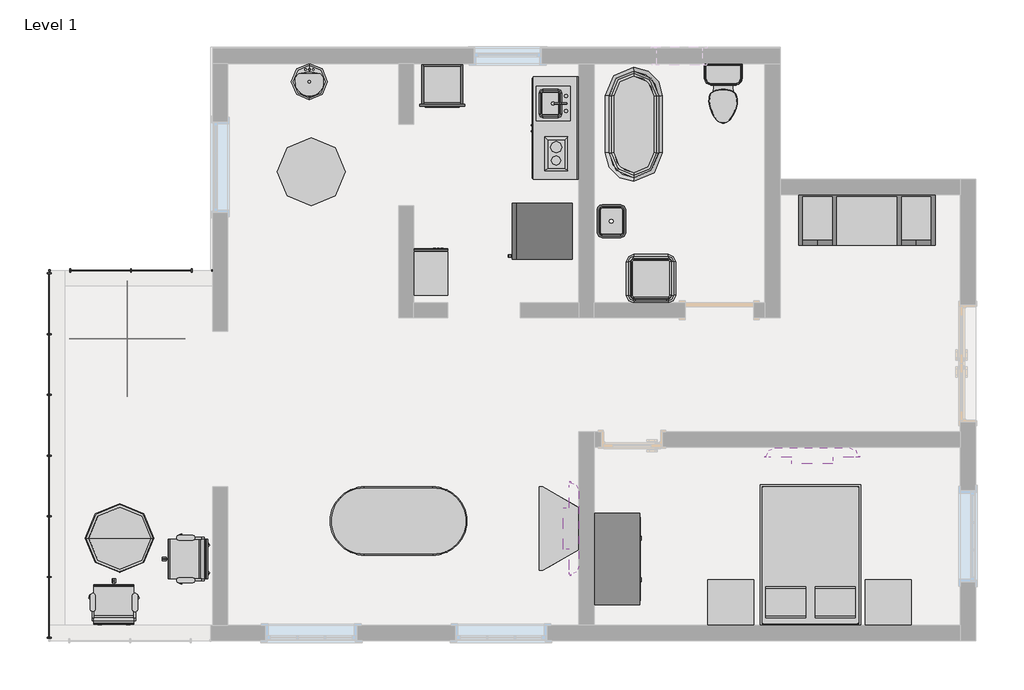
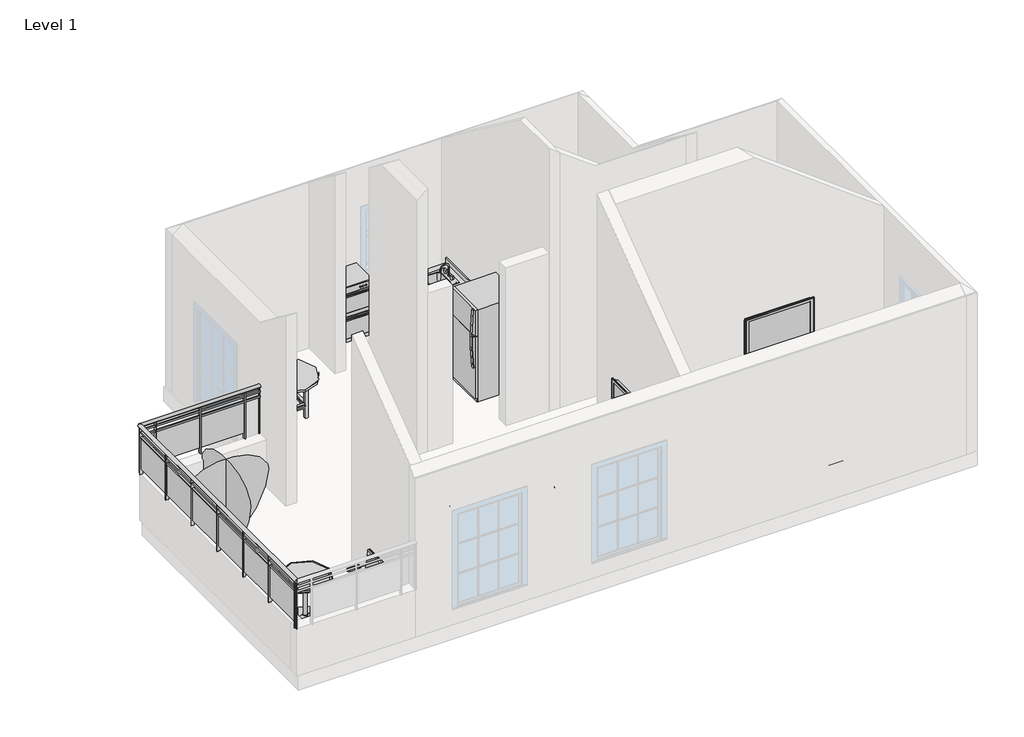
# One storey, part 2 of 2: 14 furniture elements, 5 flow terminals, 5 proxies, 2 geographic elements, 2 railings.
"""IFC4 building model written with IfcOpenShell, lengths in millimetres."""

from ifc_helpers import new_model, si_unit, point, frame, origin, place, context, project, spatial, polyline, ellipse_curve, trimmed, outline, extrude, transform, mapped, element, save
from ifc_brep_helpers import plane_surface, extruded_surface, advanced_brep
from components import proxy_7e1014cc, proxy_fe84b772, proxy_844211aa, proxy_8b8c2dc4, proxy_a13a33b2, flow_terminal_871c2e40, flow_terminal_d49f872f, flow_terminal_62a433f7, toilet_domestic_3d_toilet_domestic_3d_f7549cf7, toilet_domestic_3d_toilet_domestic_3d_183bbd19, flow_terminal_b374fae2, furniture_c8abb964, chair_task_arms_chair_task_arms_fa5a08ef, furniture_95afb093, furniture_9fa109b2, furniture_cf0b6580, furniture_fdf74506, tv_stand_tv_stand_2bc30e45, furniture_2c34a4f9, furniture_905aceb5, furniture_5bc9ed15, furniture_c80d6d9c, geographic_element_ca6e1e19, trash_can_trash_can_952d1acd

model = new_model("IFC4")

# Units and contexts
model_context = context("Model", 3, world=origin())
ifc_project = project(units=[si_unit("LENGTHUNIT", "METRE", prefix="MILLI")], contexts=[model_context])

# Site, building, storey
site = spatial("IfcSite", under=ifc_project)
building = spatial("IfcBuilding", under=site)
storey = spatial("IfcBuildingStorey", under=building, Name="Level 1", Elevation=0.0)

# Proxies
placement = place(None, origin())
proxy_shape = proxy_7e1014cc(model_context)
element("IfcBuildingElementProxy", 1, Name="18\" x 24\" x 34 1/2\"", ObjectType="18\" x 24\" x 34 1/2\"", at=placement, inside=storey, context=model_context, shape_type="MappedRepresentation", body=[
    mapped(proxy_shape, transform((-14621.294404, 11196.2948057, 0.0), x_axis=(-1.0000000000000002, 0.0, 0.0), y_axis=(0.0, -1.0000000000000002, 0.0), z_axis=(0.0, 0.0, 1.0))),
])
proxy_2_shape = proxy_fe84b772(model_context)
element("IfcBuildingElementProxy", 2, Name="Cook Top-2 Unit : 12\" x 18\"", ObjectType="Cook Top-2 Unit : 12\" x 18\"", at=placement, inside=storey, context=model_context, shape_type="MappedRepresentation", body=[
    mapped(proxy_2_shape, transform((-13327.2118725, 12487.1204454, 0.0), x_axis=(1.0, 0.0, 0.0), y_axis=(0.0, 1.0, 0.0), z_axis=(0.0, 0.0, 1.0))),
])
proxy_3_shape = proxy_844211aa(model_context)
element("IfcBuildingElementProxy", 3, Name="Kitchenette - Small : 54\"", ObjectType="Kitchenette - Small : 54\"", at=placement, inside=storey, context=model_context, shape_type="MappedRepresentation", body=[
    mapped(proxy_3_shape, transform((-12946.2118725, 12878.9829459, 0.0), x_axis=(0.0, -1.0, 0.0), y_axis=(1.0, 0.0, 0.0), z_axis=(0.0, 0.0, 1.0))),
])
proxy_4_shape = proxy_8b8c2dc4(model_context)
element("IfcBuildingElementProxy", 4, Name="Oven Double-Built-in : 21 1/2\" x 39 1/4\" x 21\"", ObjectType="Oven Double-Built-in : 21 1/2\" x 39 1/4\" x 21\"", at=placement, inside=storey, context=model_context, shape_type="MappedRepresentation", body=[
    mapped(proxy_4_shape, transform((-14739.8369452, 13303.379382, 0.0), x_axis=(1.0, 0.0, 0.0), y_axis=(0.0, 1.0, 0.0), z_axis=(0.0, 0.0, 1.0))),
])
proxy_5_shape = proxy_a13a33b2(model_context)
element("IfcBuildingElementProxy", 5, Name="Refrigerator : 30\" x 32\" RH", ObjectType="Refrigerator : 30\" x 32\" RH", at=placement, inside=storey, context=model_context, shape_type="MappedRepresentation", body=[
    mapped(proxy_5_shape, transform((-13420.8743725, 11481.0962695, 0.0), x_axis=(0.0, -1.0000000000000007, 0.0), y_axis=(1.0000000000000007, 0.0, 0.0), z_axis=(0.0, 0.0, 1.0))),
])

# Flow terminals
flow_terminal_shape = flow_terminal_871c2e40(model_context)
element("IfcFlowTerminal", 6, ObjectType="Sink Kitchen-Island : 18\" x 18\"", at=placement, inside=storey, context=model_context, shape_type="MappedRepresentation", body=[
    mapped(flow_terminal_shape, transform((-13291.4572736, 13206.1344815, 0.0), x_axis=(0.0, -1.0, 0.0), y_axis=(1.0, 0.0, 0.0), z_axis=(0.0, 0.0, 1.0))),
])
flow_terminal_2_shape = flow_terminal_d49f872f(model_context)
element("IfcFlowTerminal", 7, ObjectType="Sink Vanity-Round : 19\" x 19\"", at=placement, inside=storey, context=model_context, shape_type="MappedRepresentation", body=[
    mapped(flow_terminal_2_shape, transform((-16649.6636131, 13397.593704, 304.8), x_axis=(1.0, 0.0, 0.0), y_axis=(0.0, 1.0, 0.0), z_axis=(0.0, 0.0, 1.0))),
])
flow_terminal_3_shape = flow_terminal_62a433f7(model_context)
element("IfcFlowTerminal", 8, ObjectType="Sink Vanity-Square : 20\" x 18\"", at=placement, inside=storey, context=model_context, shape_type="MappedRepresentation", body=[
    mapped(flow_terminal_3_shape, transform((-12562.8664714, 11599.9560004, 609.6), x_axis=(0.0, 1.0, 0.0), y_axis=(-1.0, 0.0, 0.0), z_axis=(0.0, 0.0, 1.0))),
])
toilet_domestic_3d_toilet_domestic_3d_shape = toilet_domestic_3d_toilet_domestic_3d_f7549cf7(model_context)
toilet_domestic_3d_toilet_domestic_3d_2_shape = toilet_domestic_3d_toilet_domestic_3d_183bbd19(model_context)
element("IfcFlowTerminal", 9, ObjectType="Toilet-Domestic-3D : Toilet-Domestic-3D", at=placement, inside=storey, context=model_context, shape_type="MappedRepresentation", body=[
    mapped(toilet_domestic_3d_toilet_domestic_3d_shape, transform((-11015.8118725, 13229.1492136, 0.0), x_axis=(1.0, 0.0, 0.0), y_axis=(0.0, 1.0, 0.0), z_axis=(0.0, 0.0, 1.0))),
    mapped(toilet_domestic_3d_toilet_domestic_3d_2_shape, transform((-11015.8118725, 13229.1492136, 0.0), x_axis=(1.0, 0.0, 0.0), y_axis=(0.0, 1.0, 0.0), z_axis=(0.0, 0.0, 1.0))),
])
flow_terminal_4_shape = flow_terminal_b374fae2(model_context)
element("IfcFlowTerminal", 10, ObjectType="Tub-Free Standing-3D : 30\" x 60\"", at=placement, inside=storey, context=model_context, shape_type="MappedRepresentation", body=[
    mapped(flow_terminal_4_shape, transform((-12209.6118725, 12911.0452409, 0.0), x_axis=(1.0, 0.0, 0.0), y_axis=(0.0, 1.0, 0.0), z_axis=(0.0, 0.0, 1.0))),
])

# Furniture
furniture_shape = furniture_c8abb964(model_context)
element("IfcFurniture", 11, ObjectType="Bed-Box : Double 53\" x 74\"", at=placement, inside=storey, context=model_context, shape_type="MappedRepresentation", body=[
    mapped(furniture_shape, transform((-9508.2594135, 6910.8157327, 0.0), x_axis=(-1.0, 0.0, 0.0), y_axis=(0.0, -1.0, 0.0), z_axis=(0.0, 0.0, 1.0))),
])
chair_task_arms_chair_task_arms_shape = chair_task_arms_chair_task_arms_fa5a08ef(model_context)
element("IfcFurniture", 12, ObjectType="Chair-Task Arms : Chair-Task Arms", at=placement, inside=storey, context=model_context, shape_type="MappedRepresentation", body=[
    mapped(chair_task_arms_chair_task_arms_shape, transform((-18159.6659709, 6953.4544213, 0.0), x_axis=(0.0, 1.0000000000000009, 0.0), y_axis=(-1.0000000000000009, 0.0, 0.0), z_axis=(0.0, 0.0, 1.0))),
])
element("IfcFurniture", 13, ObjectType="Chair-Task Arms : Chair-Task Arms", at=placement, inside=storey, context=model_context, shape_type="MappedRepresentation", body=[
    mapped(chair_task_arms_chair_task_arms_shape, transform((-19310.2026922, 6465.8993393, 0.0), x_axis=(1.0000000000000009, 0.0, 0.0), y_axis=(0.0, 1.0000000000000009, 0.0), z_axis=(0.0, 0.0, 1.0))),
])
furniture_2_shape = furniture_95afb093(model_context)
element("IfcFurniture", 14, ObjectType="Counter Top w Sink Hole : 24\" Depth", at=placement, inside=storey, context=model_context, shape_type="MappedRepresentation", body=[
    mapped(furniture_2_shape, transform((-12946.2118725, 12345.5829459, 0.0), x_axis=(0.0, -1.0, 0.0), y_axis=(1.0, 0.0, 0.0), z_axis=(0.0, 0.0, 1.0))),
])
furniture_3_shape = furniture_9fa109b2(model_context)
element("IfcFurniture", 15, ObjectType="Dresser : 48\" x 72\" x 24\"", at=placement, inside=storey, context=model_context, shape_type="MappedRepresentation", body=[
    mapped(furniture_3_shape, transform((-12801.3748266, 7363.6385008, 0.0), x_axis=(0.0, 1.0, 0.0), y_axis=(-1.0, 0.0, 0.0), z_axis=(0.0, 0.0, 1.0))),
])
furniture_4_shape = furniture_cf0b6580(model_context)
element("IfcFurniture", 16, ObjectType="Entertainment Center : 72\" x 72\" x 24\"", at=placement, inside=storey, context=model_context, shape_type="MappedRepresentation", body=[
    mapped(furniture_4_shape, transform((-9092.5355216, 12072.8452409, 0.0), x_axis=(1.0, 0.0, 0.0), y_axis=(0.0, 1.0, 0.0), z_axis=(0.0, 0.0, 1.0))),
])
furniture_5_shape = furniture_fdf74506(model_context)
element("IfcFurniture", 17, ObjectType="TV - Flat Screen : 50\"", at=placement, inside=storey, context=model_context, shape_type="MappedRepresentation", body=[
    mapped(furniture_5_shape, transform((-13004.7504962, 7496.9007268, 1219.2), x_axis=(0.0, -1.0, 0.0), y_axis=(1.0, 0.0, 0.0), z_axis=(0.0, 0.0, 1.0))),
])
element("IfcFurniture", 18, ObjectType="TV - Flat Screen : 50\"", at=placement, inside=storey, context=model_context, shape_type="MappedRepresentation", body=[
    mapped(furniture_5_shape, transform((-9818.5037656, 8522.7310093, 1219.2), x_axis=(1.0000000000000002, 0.0, 0.0), y_axis=(0.0, 1.0000000000000002, 0.0), z_axis=(0.0, 0.0, 1.0))),
])
tv_stand_tv_stand_shape = tv_stand_tv_stand_2bc30e45(model_context)
element("IfcFurniture", 19, ObjectType="TV Stand : TV Stand", at=placement, inside=storey, context=model_context, shape_type="MappedRepresentation", body=[
    mapped(tv_stand_tv_stand_shape, transform((-12946.2118725, 7626.033243, 0.0), x_axis=(0.0, -1.0000000000000004, 0.0), y_axis=(1.0000000000000004, 0.0, 0.0), z_axis=(0.0, 0.0, 1.0))),
])
furniture_6_shape = furniture_2c34a4f9(model_context)
element("IfcFurniture", 20, ObjectType="Table-Dining Oval : 36\" x 72\"", at=placement, inside=storey, context=model_context, shape_type="MappedRepresentation", body=[
    mapped(furniture_6_shape, transform((-14957.3922004, 7960.5436016, 0.0), x_axis=(1.0, 0.0, 0.0), y_axis=(0.0, 1.0, 0.0), z_axis=(0.0, 0.0, 1.0))),
])
furniture_7_shape = furniture_905aceb5(model_context)
element("IfcFurniture", 21, ObjectType="Table-Dining Round w Chairs : 36\" Diameter", at=placement, inside=storey, context=model_context, shape_type="MappedRepresentation", body=[
    mapped(furniture_7_shape, transform((-16631.2938397, 12460.9239295, 0.0), x_axis=(1.0, 0.0, 0.0), y_axis=(0.0, 1.0, 0.0), z_axis=(0.0, 0.0, 1.0))),
])
furniture_8_shape = furniture_5bc9ed15(model_context)
element("IfcFurniture", 22, ObjectType="Table-Night Stand : 24\" x 24\" x 30\"", at=placement, inside=storey, context=model_context, shape_type="MappedRepresentation", body=[
    mapped(furniture_8_shape, transform((-9114.5455028, 6205.4452409, 0.0), x_axis=(1.0, 0.0, 0.0), y_axis=(0.0, 1.0, 0.0), z_axis=(0.0, 0.0, 1.0))),
])
element("IfcFurniture", 23, ObjectType="Table-Night Stand : 24\" x 24\" x 30\"", at=placement, inside=storey, context=model_context, shape_type="MappedRepresentation", body=[
    mapped(furniture_8_shape, transform((-11222.7455028, 6205.4452409, 0.0), x_axis=(1.0, 0.0, 0.0), y_axis=(0.0, 1.0, 0.0), z_axis=(0.0, 0.0, 1.0))),
])
furniture_9_shape = furniture_c80d6d9c(model_context)
element("IfcFurniture", 24, ObjectType="Table-Round : 36\" Diameter", at=placement, inside=storey, context=model_context, shape_type="MappedRepresentation", body=[
    mapped(furniture_9_shape, transform((-19093.0118725, 7373.8452409, 0.0), x_axis=(1.0, 0.0, 0.0), y_axis=(0.0, 1.0, 0.0), z_axis=(0.0, 0.0, 1.0))),
])

# Geographic elements
geographic_element_shape = geographic_element_ca6e1e19(model_context)
element("IfcGeographicElement", 25, ObjectType="RPC Shrub : Burning Bush 4'-6\"", at=placement, inside=storey, context=model_context, shape_type="MappedRepresentation", body=[
    mapped(geographic_element_shape, transform((-18991.4118725, 10040.8452409, 0.0), x_axis=(0.0, 1.000000000000001, 0.0), y_axis=(-1.000000000000001, 0.0, 0.0), z_axis=(0.0, 0.0, 1.0))),
])
trash_can_trash_can_shape = trash_can_trash_can_952d1acd(model_context)
element("IfcGeographicElement", 26, ObjectType="Trash Can : Trash Can", at=placement, inside=storey, context=model_context, shape_type="MappedRepresentation", body=[
    mapped(trash_can_trash_can_shape, transform((-11981.0118725, 10853.6452409, 0.0), x_axis=(1.0, 0.0, 0.0), y_axis=(0.0, 1.0, 0.0), z_axis=(0.0, 0.0, 1.0))),
])

# Railings
element("IfcRailing", 27, ObjectType="Glass Panel - Bottom Fill", at=placement, inside=storey, context=model_context, shape_type="SolidModel", body=[
    advanced_brep(
    [(-20070.9118725, 6002.2452409, 1828.8), (-19994.7118725, 6002.2452409, 1828.8), (-20070.9118725, 10955.2452409, 1828.8), (-19994.7118725, 10955.2452409, 1828.8)],
    [
        (0, 1, ellipse_curve(frame((-20032.8118725, 6002.2452409, 1828.8), z_axis=(0.0, -1.0, 0.0), x_axis=(1.0, 0.0, 0.0)), 38.1, 28.575)),
        (1, 0, ellipse_curve(frame((-20032.8118725, 6002.2452409, 1828.8), z_axis=(0.0, -1.0, 0.0), x_axis=(1.0, 0.0, 0.0)), 38.1, 28.575)),
        (2, 3, ellipse_curve(frame((-20032.8118725, 10955.2452409, 1828.8), z_axis=(0.0, 1.0, 0.0), x_axis=(1.0, 0.0, 0.0)), 38.1, 28.575)),
        (3, 2, ellipse_curve(frame((-20032.8118725, 10955.2452409, 1828.8), z_axis=(0.0, 1.0, 0.0), x_axis=(1.0, 0.0, 0.0)), 38.1, 28.575)),
        (0, 2),
        (3, 1),
    ],
    [
        plane_surface(frame((-20032.8118725, 6002.2452409, 1828.8), z_axis=(0.0, -1.0, 0.0), x_axis=(0.0, 0.0, 1.0))),
        plane_surface(frame((-20032.8118725, 10955.2452409, 1828.8), z_axis=(0.0, 1.0, 0.0), x_axis=(0.0, 0.0, 1.0))),
        extruded_surface(trimmed(ellipse_curve(frame((-20032.8118725, 10955.2452409, 1828.8), z_axis=(0.0, -1.0, 0.0), x_axis=(1.0, 0.0, 0.0)), 38.1, 28.575), [point((-20070.9118725, 10955.2452409, 1828.8))], [point((-19994.7118725, 10955.2452409, 1828.8))], True, "CARTESIAN"), (0.0, -4953.0, 0.0), 4953.0),
        extruded_surface(trimmed(ellipse_curve(frame((-20032.8118725, 10955.2452409, 1828.8), z_axis=(0.0, -1.0, 0.0), x_axis=(1.0, 0.0, 0.0)), 38.1, 28.575), [point((-19994.7118725, 10955.2452409, 1828.8))], [point((-20070.9118725, 10955.2452409, 1828.8))], True, "CARTESIAN"), (0.0, -4953.0, 0.0), 4953.0),
    ],
    [
        (0, [[1, 2]]),
        (1, [[3, 4]]),
        (2, [[-1, 5, -4, 6]]),
        (3, [[-2, -6, -3, -5]]),
    ],
),
    extrude(outline(polyline([(-20020.1118725, 6002.2452409), (-20045.5118725, 6002.2452409), (-20045.5118725, 10955.2452409), (-20020.1118725, 10955.2452409), (-20020.1118725, 6002.2452409)])), frame((0.0, 0.0, 1714.5), z_axis=(0.0, 0.0, 1.0), x_axis=(1.0, 0.0, 0.0)), (0.0, 0.0, 1.0), 25.4),
    extrude(outline(polyline([(-20020.1118725, 6002.2452409), (-20045.5118725, 6002.2452409), (-20045.5118725, 10955.2452409), (-20020.1118725, 10955.2452409), (-20020.1118725, 6002.2452409)])), frame((0.0, 0.0, 1612.9), z_axis=(0.0, 0.0, 1.0), x_axis=(1.0, 0.0, 0.0)), (0.0, 0.0, 1.0), 25.4),
    extrude(outline(polyline([(-20007.4118725, 10910.7952409), (-20058.2118725, 10910.7952409), (-20058.2118725, 10923.4952409), (-20007.4118725, 10923.4952409), (-20007.4118725, 10910.7952409)])), frame((0.0, 0.0, 914.4), z_axis=(0.0, 0.0, 1.0), x_axis=(1.0, 0.0, 0.0)), (0.0, 0.0, 1.0), 885.6788223),
    extrude(outline(polyline([(-20039.3470295, 10104.3452409), (-20039.3470295, 10917.1452409), (-20032.9970295, 10917.1452409), (-20032.9970295, 10104.3452409), (-20039.3470295, 10104.3452409)])), frame((0.0, 0.0, 1016.0), z_axis=(0.0, 0.0, 1.0), x_axis=(1.0, 0.0, 0.0)), (0.0, 0.0, 1.0), 596.9),
    extrude(outline(polyline([(-20007.4118725, 10097.9952409), (-20058.2118725, 10097.9952409), (-20058.2118725, 10110.6952409), (-20007.4118725, 10110.6952409), (-20007.4118725, 10097.9952409)])), frame((0.0, 0.0, 914.4), z_axis=(0.0, 0.0, 1.0), x_axis=(1.0, 0.0, 0.0)), (0.0, 0.0, 1.0), 885.6788223),
    extrude(outline(polyline([(-20039.3470295, 9291.5452409), (-20039.3470295, 10104.3452409), (-20032.9970295, 10104.3452409), (-20032.9970295, 9291.5452409), (-20039.3470295, 9291.5452409)])), frame((0.0, 0.0, 1016.0), z_axis=(0.0, 0.0, 1.0), x_axis=(1.0, 0.0, 0.0)), (0.0, 0.0, 1.0), 596.9),
    extrude(outline(polyline([(-20007.4118725, 9285.1952409), (-20058.2118725, 9285.1952409), (-20058.2118725, 9297.8952409), (-20007.4118725, 9297.8952409), (-20007.4118725, 9285.1952409)])), frame((0.0, 0.0, 914.4), z_axis=(0.0, 0.0, 1.0), x_axis=(1.0, 0.0, 0.0)), (0.0, 0.0, 1.0), 885.6788223),
    extrude(outline(polyline([(-20039.3470295, 8478.7452409), (-20039.3470295, 9291.5452409), (-20032.9970295, 9291.5452409), (-20032.9970295, 8478.7452409), (-20039.3470295, 8478.7452409)])), frame((0.0, 0.0, 1016.0), z_axis=(0.0, 0.0, 1.0), x_axis=(1.0, 0.0, 0.0)), (0.0, 0.0, 1.0), 596.9),
    extrude(outline(polyline([(-20007.4118725, 8472.3952409), (-20058.2118725, 8472.3952409), (-20058.2118725, 8485.0952409), (-20007.4118725, 8485.0952409), (-20007.4118725, 8472.3952409)])), frame((0.0, 0.0, 914.4), z_axis=(0.0, 0.0, 1.0), x_axis=(1.0, 0.0, 0.0)), (0.0, 0.0, 1.0), 885.6788223),
    extrude(outline(polyline([(-20039.3470295, 7665.9452409), (-20039.3470295, 8478.7452409), (-20032.9970295, 8478.7452409), (-20032.9970295, 7665.9452409), (-20039.3470295, 7665.9452409)])), frame((0.0, 0.0, 1016.0), z_axis=(0.0, 0.0, 1.0), x_axis=(1.0, 0.0, 0.0)), (0.0, 0.0, 1.0), 596.9),
    extrude(outline(polyline([(-20007.4118725, 7659.5952409), (-20058.2118725, 7659.5952409), (-20058.2118725, 7672.2952409), (-20007.4118725, 7672.2952409), (-20007.4118725, 7659.5952409)])), frame((0.0, 0.0, 914.4), z_axis=(0.0, 0.0, 1.0), x_axis=(1.0, 0.0, 0.0)), (0.0, 0.0, 1.0), 885.6788223),
    extrude(outline(polyline([(-20039.3470295, 6853.1452409), (-20039.3470295, 7665.9452409), (-20032.9970295, 7665.9452409), (-20032.9970295, 6853.1452409), (-20039.3470295, 6853.1452409)])), frame((0.0, 0.0, 1016.0), z_axis=(0.0, 0.0, 1.0), x_axis=(1.0, 0.0, 0.0)), (0.0, 0.0, 1.0), 596.9),
    extrude(outline(polyline([(-20007.4118725, 6846.7952409), (-20058.2118725, 6846.7952409), (-20058.2118725, 6859.4952409), (-20007.4118725, 6859.4952409), (-20007.4118725, 6846.7952409)])), frame((0.0, 0.0, 914.4), z_axis=(0.0, 0.0, 1.0), x_axis=(1.0, 0.0, 0.0)), (0.0, 0.0, 1.0), 885.6788223),
    extrude(outline(polyline([(-20039.3470295, 6040.3452409), (-20039.3470295, 6853.1452409), (-20032.9970295, 6853.1452409), (-20032.9970295, 6040.3452409), (-20039.3470295, 6040.3452409)])), frame((0.0, 0.0, 1016.0), z_axis=(0.0, 0.0, 1.0), x_axis=(1.0, 0.0, 0.0)), (0.0, 0.0, 1.0), 596.9),
    extrude(outline(polyline([(-20007.4118725, 6033.9952409), (-20058.2118725, 6033.9952409), (-20058.2118725, 6046.6952409), (-20007.4118725, 6046.6952409), (-20007.4118725, 6033.9952409)])), frame((0.0, 0.0, 914.4), z_axis=(0.0, 0.0, 1.0), x_axis=(1.0, 0.0, 0.0)), (0.0, 0.0, 1.0), 885.6788223),
    extrude(outline(polyline([(-20023.2868725, 10942.5452409), (-20042.3368725, 10942.5452409), (-20042.3368725, 10961.5952409), (-20023.2868725, 10961.5952409), (-20023.2868725, 10942.5452409)])), frame((0.0, 0.0, 914.4), z_axis=(0.0, 0.0, 1.0), x_axis=(1.0, 0.0, 0.0)), (0.0, 0.0, 1.0), 885.6788223),
    extrude(outline(polyline([(-20023.2868725, 5995.8952409), (-20042.3368725, 5995.8952409), (-20042.3368725, 6014.9452409), (-20023.2868725, 6014.9452409), (-20023.2868725, 5995.8952409)])), frame((0.0, 0.0, 914.4), z_axis=(0.0, 0.0, 1.0), x_axis=(1.0, 0.0, 0.0)), (0.0, 0.0, 1.0), 885.6788223),
])
element("IfcRailing", 28, ObjectType="Glass Panel - Bottom Fill", at=placement, inside=storey, context=model_context, shape_type="SolidModel", body=[
    advanced_brep(
    [(-20032.8118725, 10993.3452409, 1828.8), (-20032.8118725, 10917.1452409, 1828.8), (-17848.4118725, 10993.3452409, 1828.8), (-17848.4118725, 10917.1452409, 1828.8)],
    [
        (0, 1, ellipse_curve(frame((-20032.8118725, 10955.2452409, 1828.8), z_axis=(-1.0, 0.0, 0.0), x_axis=(0.0, -1.0, 0.0)), 38.1, 28.575)),
        (1, 0, ellipse_curve(frame((-20032.8118725, 10955.2452409, 1828.8), z_axis=(-1.0, 0.0, 0.0), x_axis=(0.0, -1.0, 0.0)), 38.1, 28.575)),
        (2, 3, ellipse_curve(frame((-17848.4118725, 10955.2452409, 1828.8), z_axis=(1.0, 0.0, 0.0), x_axis=(0.0, -1.0, 0.0)), 38.1, 28.575)),
        (3, 2, ellipse_curve(frame((-17848.4118725, 10955.2452409, 1828.8), z_axis=(1.0, 0.0, 0.0), x_axis=(0.0, -1.0, 0.0)), 38.1, 28.575)),
        (0, 2),
        (3, 1),
    ],
    [
        plane_surface(frame((-20032.8118725, 10955.2452409, 1828.8), z_axis=(-1.0, 0.0, 0.0), x_axis=(0.0, 1.0, 0.0))),
        plane_surface(frame((-17848.4118725, 10955.2452409, 1828.8), z_axis=(1.0, 0.0, 0.0), x_axis=(0.0, 1.0, 0.0))),
        extruded_surface(trimmed(ellipse_curve(frame((-17848.4118725, 10955.2452409, 1828.8), z_axis=(-1.0, 0.0, 0.0), x_axis=(0.0, -1.0, 0.0)), 38.1, 28.575), [point((-17848.4118725, 10993.3452409, 1828.8))], [point((-17848.4118725, 10917.1452409, 1828.8))], True, "CARTESIAN"), (-2184.399999999998, 0.0, 0.0), 2184.399999999998),
        extruded_surface(trimmed(ellipse_curve(frame((-17848.4118725, 10955.2452409, 1828.8), z_axis=(-1.0, 0.0, 0.0), x_axis=(0.0, -1.0, 0.0)), 38.1, 28.575), [point((-17848.4118725, 10917.1452409, 1828.8))], [point((-17848.4118725, 10993.3452409, 1828.8))], True, "CARTESIAN"), (-2184.399999999998, 0.0, 0.0), 2184.399999999998),
    ],
    [
        (0, [[1, 2]]),
        (1, [[3, 4]]),
        (2, [[-1, 5, -4, 6]]),
        (3, [[-2, -6, -3, -5]]),
    ],
),
    extrude(outline(polyline([(-20032.8118725, 10942.5452409), (-20032.8118725, 10967.9452409), (-17848.4118725, 10967.9452409), (-17848.4118725, 10942.5452409), (-20032.8118725, 10942.5452409)])), frame((0.0, 0.0, 1714.5), z_axis=(0.0, 0.0, 1.0), x_axis=(1.0, 0.0, 0.0)), (0.0, 0.0, 1.0), 25.4),
    extrude(outline(polyline([(-20032.8118725, 10942.5452409), (-20032.8118725, 10967.9452409), (-17848.4118725, 10967.9452409), (-17848.4118725, 10942.5452409), (-20032.8118725, 10942.5452409)])), frame((0.0, 0.0, 1612.9), z_axis=(0.0, 0.0, 1.0), x_axis=(1.0, 0.0, 0.0)), (0.0, 0.0, 1.0), 25.4),
    extrude(outline(polyline([(-18134.1618725, 10929.8452409), (-18134.1618725, 10980.6452409), (-18121.4618725, 10980.6452409), (-18121.4618725, 10929.8452409), (-18134.1618725, 10929.8452409)])), frame((0.0, 0.0, 914.4), z_axis=(0.0, 0.0, 1.0), x_axis=(1.0, 0.0, 0.0)), (0.0, 0.0, 1.0), 885.6788223),
    extrude(outline(polyline([(-18940.6118725, 10961.7803979), (-18127.8118725, 10961.7803979), (-18127.8118725, 10955.4303979), (-18940.6118725, 10955.4303979), (-18940.6118725, 10961.7803979)])), frame((0.0, 0.0, 1016.0), z_axis=(0.0, 0.0, 1.0), x_axis=(1.0, 0.0, 0.0)), (0.0, 0.0, 1.0), 596.9),
    extrude(outline(polyline([(-18946.9618725, 10929.8452409), (-18946.9618725, 10980.6452409), (-18934.2618725, 10980.6452409), (-18934.2618725, 10929.8452409), (-18946.9618725, 10929.8452409)])), frame((0.0, 0.0, 914.4), z_axis=(0.0, 0.0, 1.0), x_axis=(1.0, 0.0, 0.0)), (0.0, 0.0, 1.0), 885.6788223),
    extrude(outline(polyline([(-19753.4118725, 10961.7803979), (-18940.6118725, 10961.7803979), (-18940.6118725, 10955.4303979), (-19753.4118725, 10955.4303979), (-19753.4118725, 10961.7803979)])), frame((0.0, 0.0, 1016.0), z_axis=(0.0, 0.0, 1.0), x_axis=(1.0, 0.0, 0.0)), (0.0, 0.0, 1.0), 596.9),
    extrude(outline(polyline([(-19759.7618725, 10929.8452409), (-19759.7618725, 10980.6452409), (-19747.0618725, 10980.6452409), (-19747.0618725, 10929.8452409), (-19759.7618725, 10929.8452409)])), frame((0.0, 0.0, 914.4), z_axis=(0.0, 0.0, 1.0), x_axis=(1.0, 0.0, 0.0)), (0.0, 0.0, 1.0), 885.6788223),
    extrude(outline(polyline([(-17861.1118725, 10945.7202409), (-17861.1118725, 10964.7702409), (-17842.0618725, 10964.7702409), (-17842.0618725, 10945.7202409), (-17861.1118725, 10945.7202409)])), frame((0.0, 0.0, 914.4), z_axis=(0.0, 0.0, 1.0), x_axis=(1.0, 0.0, 0.0)), (0.0, 0.0, 1.0), 885.6788223),
    extrude(outline(polyline([(-20039.1618725, 10945.7202409), (-20039.1618725, 10964.7702409), (-20020.1118725, 10964.7702409), (-20020.1118725, 10945.7202409), (-20039.1618725, 10945.7202409)])), frame((0.0, 0.0, 914.4), z_axis=(0.0, 0.0, 1.0), x_axis=(1.0, 0.0, 0.0)), (0.0, 0.0, 1.0), 885.6788223),
])

save(model, "model.ifc")

# Revit data of these elements
# Type "18\" x 24\" x 34 1/2\""
#   Label = "T"
#   Assembly Code = "E1090400"
#   Depth = 2' - 0"
#   Height = 2' - 10 1/2"
#   Width = 1' - 6"
#   Panel Face Material = Plastic, Opaque Black
#   Trach Compact. Material = Steel, Paint Finish, Ivory, Matte
#   Default Elevation = 0
# Type "Cook Top-2 Unit : 12\" x 18\""
#   Assembly Code = "E1090400"
#   Counter Height = 3' - 0"
#   Depth = 1' - 6"
#   Width = 1' - 0"
#   Burner Material = Steel, Chrome Plated
#   Cooktop Material = Steel, Polished
#   Default Elevation = 0
# Type "Kitchenette - Small : 54\""
#   Assembly Code = "E1090400"
#   Width = 4' - 6"
#   Height = 2' - 10 1/2"
#   Depth = 2' - 0"
#   Toe Depth = 0' - 3"
#   Toe Height = 0' - 3 1/2"
#   Cabinet Material = Cabinets
#   Door/Drawer Material = Cabinets
#   Handle Material = Cabinets - Handles
#   Default Elevation = 0
# Type "Oven Double-Built-in : 21 1/2\" x 39 1/4\" x 21\""
#   Label = "OVEN"
#   Assembly Code = "E1090400"
#   Depth = 1' - 9"
#   Height = 3' - 3 1/4"
#   Width = 1' - 9 1/2"
#   Oven Material = Metal - Stainless Steel, Polished
#   Default Elevation = 0
# Type "Refrigerator : 30\" x 32\" RH"
#   Label = "REF."
#   Assembly Code = "E1090400"
#   Depth = 2' - 7 3/4"
#   Handle = 2' - 3"
#   Height = 5' - 10"
#   Rear Clearance = 0' - 2"
#   Top Door Height = 1' - 8"
#   Width = 2' - 5 3/8"
#   Material = Steel, Paint Finish, Ivory, Glossy
#   Default Elevation = 0
# Type "Sink Kitchen-Island : 18\" x 18\""
#   Assembly Code = "D2010410"
#   Counter Height = 3' - 0"
#   Depth = 1' - 6"
#   Width = 1' - 6"
#   Faucet Material = Steel, Polished
#   Sink Material = Steel, Polished
#   Default Elevation = 0
# Type "Sink Vanity-Round : 19\" x 19\""
#   Assembly Code = "D2010400"
#   Top Of Counter = 2' - 7"
#   Basin Material = Porcelain, Linen
#   Faucet Material = Steel, Polished
#   Default Elevation = 0
# Type "Sink Vanity-Square : 20\" x 18\""
#   Assembly Code = "D2010400"
#   Counter Height = 2' - 7"
#   Depth = 1' - 6"
#   Width = 1' - 8"
#   Basin Material = Porcelain, Linen
#   Faucet Material = Steel, Polished
#   Default Elevation = 0
# Type "Toilet-Domestic-3D : Toilet-Domestic-3D"
#   Assembly Code = "D2010110"
#   Toilet - Bowl/Basin Material = Porcelain, Linen
#   Toilet - Seat Material = Laminate, Linen, Matte
#   Default Elevation = 0
# Type "Tub-Free Standing-3D : 30\" x 60\""
#   Assembly Code = "D2010110"
#   Height = 1' - 6"
#   Length = 5' - 0"
#   Width = 2' - 6"
#   Tub Material = Porcelain, Ivory
#   Default Elevation = 0
# Type "Bed-Box : Double 53\" x 74\""
#   Assembly Code = "E2020200"
#   Length = 6' - 2"
#   Width = 4' - 5"
#   Frame Material = Birch
#   Mattress Material = Linen, White
#   Default Elevation = 0
# Type "Chair-Task Arms : Chair-Task Arms"
#   Assembly Code = "E2020200"
#   Base Material = Plastic, Opaque Black
#   Caster Material = Plastic, Opaque Black
#   Seat/Back Material = Textile - Slate Blue
#   Default Elevation = 0
# Type "Counter Top w Sink Hole : 24\" Depth"
#   Assembly Code = "C1030400"
#   Counter Thickness = 0' - 1 1/2"
#   Depth [instance default] = 2' - 1"
#   Height = 3' - 0"
#   Length [instance default] = 8' - 0"
#   Sink Location [instance default] = 2' - 0"
#   Sink Location To Wall [instance default] = 0' - 6"
#   Sink Opening Depth [instance default] = 1' - 3"
#   Sink Opening Width [instance default] = 2' - 3"
#   Counter Top Material = none
#   Default Elevation = 0
# Type "Dresser : 48\" x 72\" x 24\""
#   Assembly Code = "E2020200"
#   Depth = 2' - 0"
#   Height = 6' - 0"
#   Width = 4' - 0"
#   Dresser Material = Laminate - Ivory, Glossy
#   Drawer Material = Laminate, Ivory, Matte
#   Knob Material = Cherry
#   Default Elevation = 0
# Type "Entertainment Center : 72\" x 72\" x 24\""
#   Assembly Code = "E2020200"
#   Center Width = 2' - 8"
#   Depth = 2' - 0"
#   Height = 6' - 0"
#   Width = 6' - 0"
#   Material = none
#   Default Elevation = 0
# Type "TV - Flat Screen : 50\""
#   SinAng = 0' - 0.0193"
#   L = 3' - 7.57782"
#   H = 2' - 0.51477"
#   Thickness = 0' - 4.33071"
#   Diagonal = 4' - 2"
#   CosAng = 0' - 0.03431"
#   Stand [instance default] = yes
#   Default Elevation = 0
# Type "TV Stand : TV Stand"
#   Depth = 1' - 9"
#   Width = 3' - 8"
#   Height = 1' - 7 1/2"
#   Finish = Melamine - Gray
#   Default Elevation = 0
# Type "Table-Dining Oval : 36\" x 72\""
#   Assembly Code = "E2020200"
#   Length = 6' - 0"
#   Width = 3' - 0"
#   Base Material = Steel, Chrome Plated
#   Top Material = Glass - Clear, Grey
#   Default Elevation = 0
#   Description = (empty or 0)
# Type "Table-Dining Round w Chairs : 36\" Diameter"
#   Assembly Code = "E2020200"
#   Radius = 1' - 6"
#   Diameter = 3' - 0"
#   Height = 2' - 6"
#   Chairs = 4
#   Base Material = Pine
#   Top Material = Laminate, Linen, Matte
#   Default Elevation = 0
# Type "Table-Night Stand : 24\" x 24\" x 30\""
#   Assembly Code = "E2020200"
#   Depth = 2' - 0"
#   Height = 2' - 6"
#   Width = 2' - 0"
#   Base Material = Birch
#   Top Material = Laminate, Ivory, Matte
#   Default Elevation = 0
# Type "Table-Round : 36\" Diameter"
#   Assembly Code = "E2020200"
#   Base Radius = 0' - 10"
#   Height = 2' - 6"
#   Radius = 1' - 6"
#   Base Material = Steel, Chrome Plated
#   Top Material = Birch
#   Default Elevation = 0
# Type "RPC Shrub : Burning Bush 4'-6\""
#   Type Comments = "Burning Bush"
#   built-in parameter 1005198 = "{2, 15},{39, RPC-16-FVGW-0UXX-7JA7-N000-ST1L-LVER-AU},{1, 0},{1, 0},{2, 13},{1, 8},{5, Color},{1, 0},{1, 0},{3, 0.8},{3, 0.8},{3, 0.8},{1, 8},{7, BBoxMin},{1, 0},{1, 0},{1, 0},{1, 0},{1, 0},{1, 8},{7, BBoxMax},{1, 0},{1, 0},{1, 0},{1, 0},{1, 0},{2, 11},{9, RPCTypeId},{1, 0},{1, 0},{39, RPC-16-FVGW-0UXX-7JA7-N000-ST1L-LVER-AU},{1, 6},{14, RPCPlantHeight},{1, 0},{1, 0},{3, 4.5},{2, 11},{7, keyword},{1, 0},{1, 0},{35, :RPCs:Shrubs & Grasses:Geometry:RPC},{2, 11},{8, category},{1, 0},{1, 0},{16, Shrubs & Grasses},{2, 11},{12, LocalizedUID},{1, 0},{1, 0},{12, Burning Bush},{2, 14},{6, Height},{1, 0},{1, 0},{3, 4.5},{1, 2},{16, Cast Reflections},{1, 0},{1, 0},{1, 0},{1, 2},{12, Cast Shadows},{1, 0},{1, 0},{1, 1},{1, 2},{9, Lock View},{1, 0},{1, 0},{1, 0},{1, 4},{5, ViewC},{1, 0},{1, 0},{1, 0},{21, assetlibrary_base.fbx},{1, 5},"
#   built-in parameter 1005195 = "RPC-16-FVGW-0UXX-7JA7-N000-ST1L-LVER-AU"
#   Assembly Code = "G2050500"
#   Height = 4' - 6"
#   Default Elevation = 0
# Type "Trash Can : Trash Can"
#   Assembly Code = "G2040900"
# Type "Glass Panel - Bottom Fill"
#   Assembly Code = "C2010400"
#   built-in parameter 1008612 = 0.0416667 (stored number, unit not read)
#   built-in parameter 1008611 = 0.0416667 (stored number, unit not read)
#   built-in parameter 1008609 = 0.333333 (stored number, unit not read)
#   built-in parameter 1008604 = 0.166667 (stored number, unit not read)
#   built-in parameter 1008603 = 0.166667 (stored number, unit not read)
#   Railing Height = 3' - 0"
#   built-in parameter 1008630 = 2
#   built-in parameter 1008610 = 2
#   built-in parameter 1008618 = Baluster - Square : 3/4"
# Element 1 (IfcBuildingElementProxy, "18\" x 24\" x 34 1/2\"")
#   Phase Created = New Construction
#   Materials on its faces: "Steel, Paint Finish, Ivory, Matte", "Plastic, Opaque Black"
# Element 2 (IfcBuildingElementProxy, "Cook Top-2 Unit : 12\" x 18\"")
#   Phase Created = New Construction
#   Materials on its faces: "Steel, Chrome Plated", "Steel, Polished"
# Element 3 (IfcBuildingElementProxy, "Kitchenette - Small : 54\"")
#   Phase Created = New Construction
#   Materials on its faces: "Cabinets", "Cabinets - Handles"
# Element 4 (IfcBuildingElementProxy, "Oven Double-Built-in : 21 1/2\" x 39 1/4\" x 21\"")
#   Phase Created = New Construction
#   Materials on its faces: "Steel", "Metal - Stainless Steel, Polished", "Glass"
# Element 5 (IfcBuildingElementProxy, "Refrigerator : 30\" x 32\" RH")
#   Phase Created = New Construction
#   Materials on its faces: "Steel, Paint Finish, Ivory, Glossy", "Steel, Chrome Plated"
# Element 6 (IfcFlowTerminal, "Sink Kitchen-Island : 18\" x 18\"")
#   Mark = "1"
#   Phase Created = New Construction
#   Materials on its faces: "Steel, Polished"
# Element 7 (IfcFlowTerminal, "Sink Vanity-Round : 19\" x 19\"")
#   Mark = "6"
#   Phase Created = New Construction
#   Materials on its faces: "Porcelain, Linen", "Steel, Polished"
# Element 8 (IfcFlowTerminal, "Sink Vanity-Square : 20\" x 18\"")
#   Mark = "5"
#   Phase Created = New Construction
#   Materials on its faces: "Porcelain, Linen", "Steel, Polished"
# Element 9 (IfcFlowTerminal, "Toilet-Domestic-3D : Toilet-Domestic-3D")
#   Mark = "4"
#   Phase Created = New Construction
#   Materials on its faces: "Porcelain, Linen", "Laminate, Linen, Matte"
# Element 10 (IfcFlowTerminal, "Tub-Free Standing-3D : 30\" x 60\"")
#   Mark = "2"
#   Phase Created = New Construction
#   Materials on its faces: "Porcelain, Ivory"
# Element 11 (IfcFurniture, "Bed-Box : Double 53\" x 74\"")
#   Phase Created = New Construction
#   Materials on its faces: "Birch", "Linen, White"
# Elements 12, 13 (IfcFurniture, "Chair-Task Arms : Chair-Task Arms")
#   Phase Created = New Construction
#   Materials on its faces: "Plastic, Opaque Black", "Textile - Slate Blue"
# Element 14 (IfcFurniture, "Counter Top w Sink Hole : 24\" Depth")
#   Sink Opening Depth = 1' - 3"
#   Sink Location To Wall = 0' - 6"
#   Length = 4' - 6"
#   Sink Location = 1' - 2"
#   Sink Opening Width = 1' - 4"
#   Depth = 2' - 0"
#   Phase Created = New Construction
#   Materials on its faces: "Counter Top"
# Element 15 (IfcFurniture, "Dresser : 48\" x 72\" x 24\"")
#   Phase Created = New Construction
#   Materials on its faces: "Laminate, Ivory, Matte", "Cherry", "Laminate - Ivory, Glossy"
# Element 16 (IfcFurniture, "Entertainment Center : 72\" x 72\" x 24\"")
#   Phase Created = New Construction
#   Materials on its faces: "Steel, Chrome Plated", "Glass - Clear, Grey"
# Elements 17, 18 (IfcFurniture, "TV - Flat Screen : 50\"")
#   Stand = yes
#   Phase Created = New Construction
#   Materials on its faces: "TV - Black", "TV - Glass", "TV - Screen"
# Element 19 (IfcFurniture, "TV Stand : TV Stand")
#   Phase Created = New Construction
#   Materials on its faces: "Melamine - Gray", "Glass - Shelves"
# Element 20 (IfcFurniture, "Table-Dining Oval : 36\" x 72\"")
#   Phase Created = New Construction
#   Materials on its faces: "Steel, Chrome Plated", "Glass - Clear, Grey"
# Element 21 (IfcFurniture, "Table-Dining Round w Chairs : 36\" Diameter")
#   Phase Created = New Construction
#   Materials on its faces: "Pine", "Laminate, Linen, Matte"
# Elements 22, 23 (IfcFurniture, "Table-Night Stand : 24\" x 24\" x 30\"")
#   Phase Created = New Construction
#   Materials on its faces: "Birch", "Laminate, Ivory, Matte"
# Element 24 (IfcFurniture, "Table-Round : 36\" Diameter")
#   Phase Created = New Construction
#   Materials on its faces: "Steel, Chrome Plated", "Birch"
# Element 25 (IfcGeographicElement, "RPC Shrub : Burning Bush 4'-6\"")
#   Phase Created = New Construction
# Element 26 (IfcGeographicElement, "Trash Can : Trash Can")
#   Phase Created = New Construction
#   Materials on its faces: "Plastic - Gray, Dark", "Plastic, Opaque Black"
# Elements 27, 28 (IfcRailing, "Glass Panel - Bottom Fill")
#   built-in parameter 1008621 = 3 (stored number, unit not read)
#   Phase Created = New Construction
#   Materials on its faces: "Glass"
# Materials
#   "Plastic, Opaque Black": class "Plastic", colour RGB 0 0 0, transparency 0.7, Description = "Plastic, generic, opaque black", Cost = 0
#   "Steel, Paint Finish, Ivory, Matte": class "Metal", colour RGB 247 247 239, transparency 0, Description = "Steel, paint finish, ivory, matte", Cost = 0
#   "Steel, Chrome Plated": class "Metal", colour RGB 17 17 17, transparency 0, Description = "Chromiuim plated steel", Cost = 0
#   "Steel, Polished": class "Metal", colour RGB 57 57 57, transparency 0, Description = "Polished steel", Cost = 0
#   "Cabinets": colour RGB 249 249 249, transparency 0
#   "Cabinets - Handles": class "Metal", colour RGB 57 57 57, transparency 0
#   "Metal - Stainless Steel, Polished": class "Metal", colour RGB 216 216 216, transparency 0
#   "Steel, Paint Finish, Ivory, Glossy": class "Metal", colour RGB 247 247 239, transparency 0, Description = "Steel, paint finish, ivory, glossy", Cost = 0
#   "Porcelain, Linen": class "Ceramic", colour RGB 249 239 230, transparency 0, Description = "Porcelain, linen", Cost = 0
#   "Laminate, Linen, Matte": class "Plastic", colour RGB 249 239 230, transparency 0, Description = "Plastic Laminate - Linen, Matte", Cost = 0
#   "Porcelain, Ivory": class "Ceramic", colour RGB 247 247 239, transparency 0, Description = "Porcelain, ivory", Cost = 0
#   "Birch": class "Wood", colour RGB 224 178 126, transparency 0, Description = "Betula Alleghaniensis", Cost = 0
#   "Linen, White": class "Textile", colour RGB 247 247 239, transparency 0, Description = "Linen, white", Cost = 0
#   "Textile - Slate Blue": class "Fabric", colour RGB 98 102 118, transparency 0
#   "Laminate - Ivory, Glossy": colour RGB 247 247 239, transparency 0
#   "Laminate, Ivory, Matte": class "Plastic", colour RGB 247 247 239, transparency 0, Description = "Plastic Laminate - Ivory, Matte", Cost = 0
#   "Cherry": class "Wood", colour RGB 226 177 128, transparency 0, Description = "Prunus Serotina", Cost = 0
#   "Melamine - Gray": class "Wood", colour RGB 49 49 49, transparency 0
#   "Glass - Clear, Grey": class "Glass", colour RGB 252 255 255, transparency 0.64
#   "Pine": class "Wood", colour RGB 223 192 134, transparency 0, Description = "Pinus Echinata", Cost = 0
#   "Steel": class "Metal", colour RGB 247 247 247, transparency 0, Description = "Steel, mill finish", Cost = 0
#   "Glass": class "Glass", colour RGB 0 128 192, transparency 0.75, Description = "Soda Lime Glass", Cost = 0
#   "Counter Top": class "Wood", colour RGB 226 177 128, transparency 0
#   "TV - Black": colour RGB 49 49 49, transparency 0
#   "TV - Glass": colour RGB 157 157 157, transparency 0.9
#   "TV - Screen": colour RGB 0 0 0, transparency 0
#   "Glass - Shelves": class "Glass", colour RGB 167 167 167, transparency 0.9
#   "Plastic - Gray, Dark": class "Plastic", colour RGB 134 134 134, transparency 0
